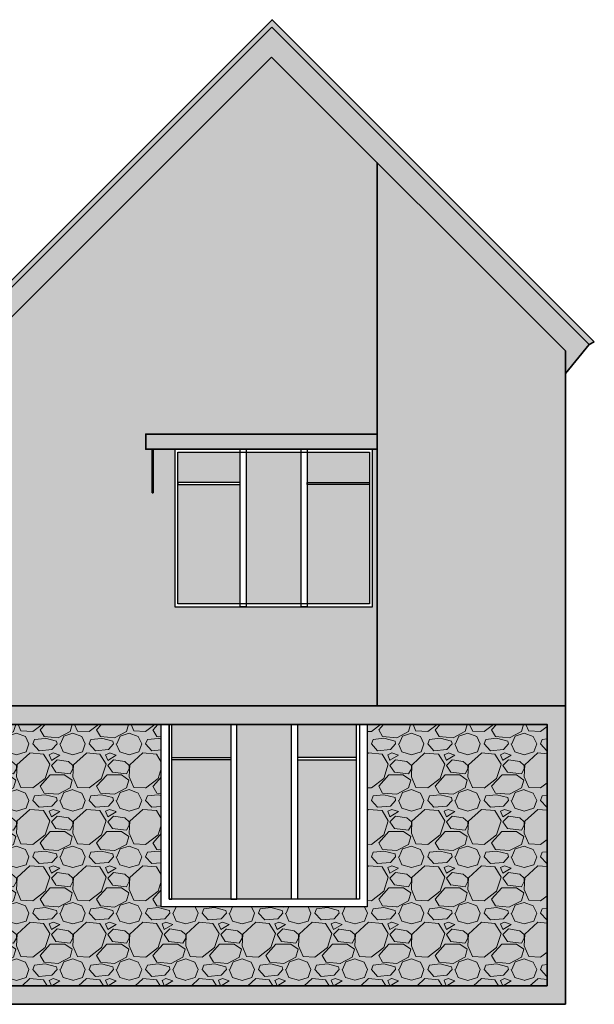
# Model space of a CAD drawing. Units: feet. Extents: x 2613 to 3913, y 950 to 1393.
# Tile 5 of 6: x 2948 to 3207, y 950 to 1393. Entities that reach past the tile are written whole.
import ezdxf

# ---------------------------------------------------------------- set-up
doc = ezdxf.new("R2010")
doc.units = ezdxf.units.FT
for name, color, linetype, lineweight in [('A-ELEV', 7, 'Continuous', 35), ('A-ELEV-PATT', 9, 'Continuous', 13), ('A-FLOR-STRS', 7, 'Continuous', 25), ('A-GLAZ', 4, 'Continuous', 25), ('A-ROOF', 1, 'Continuous', 35)]:
    doc.layers.add(name, color=color, linetype=linetype, lineweight=lineweight)

msp = doc.modelspace()

# ---------------------------------------------------------------- hatches: boundary and pattern name
at = {"layer": 'A-ELEV-PATT'}
h = msp.add_hatch(color=256, dxfattribs=at)
h.dxf.hatch_style = 1
h.paths.add_polyline_path([(3108.91, 1328.81), (3061.44, 1376.28), (2929.45, 1244.29), (2929.45, 1223.38), (2942.09, 1223.38), (2942.09, 1215.5), (2929.45, 1215.5), (2929.45, 1084.12), (3108.91, 1084.12), (3108.91, 1199.69), (3106.87, 1199.69), (3106.87, 1128.72), (3017.91, 1128.72), (3017.91, 1199.69), (3008.08, 1199.69), (3008.08, 1180.01), (3007.65, 1180.01), (3007.65, 1199.69), (3004.75, 1199.69), (3004.75, 1206.47), (3108.91, 1206.47)])
h.paths.add_polyline_path([(3061.44, 1376.28), (3193.8, 1243.92), (3193.8, 1233.84), (3204.34, 1246.9), (3061.54, 1389.71), (2918.82, 1247), (2929.45, 1233.69), (2929.45, 1244.29)])
h.paths.add_polyline_path([(3061.54, 1389.71), (3204.34, 1246.9), (3206.69, 1248.02), (3061.63, 1393.09), (2916.59, 1248.06), (2918.82, 1247)])
h.paths.add_polyline_path([(2925.65, 1257.12), (2667.59, 1257.12), (2651.33, 1257.12), (2651.33, 1252.28), (2920.82, 1252.28)])
h.paths.add_polyline_path([(2920.82, 1252.28), (2651.33, 1252.28, -0.144454), (2652.15, 1251.12), (2667.59, 1251.12), (2919.65, 1251.12)])
h.paths.add_polyline_path([(2918.82, 1247), (2916.59, 1248.06), (2919.65, 1251.12), (2667.59, 1251.12), (2652.15, 1251.12), (2667.59, 1229.14), (2667.59, 1233.69), (2929.45, 1233.69)])
h.paths.add_polyline_path([(2710.6, 1223.38), (2929.45, 1223.38), (2929.45, 1233.69), (2667.59, 1233.69), (2667.59, 1229.14), (2667.59, 1201.16), (2720.67, 1201.16), (2710.6, 1215.5)])
h.paths.add_polyline_path([(2942.09, 1223.38), (2710.6, 1223.38), (2710.6, 1215.5), (2921.48, 1215.5), (2942.09, 1215.5)])
h.paths.add_polyline_path([(2929.45, 1215.5), (2921.48, 1215.5), (2710.6, 1215.5), (2733.47, 1182.94), (2733.47, 1195.74), (2741.22, 1195.74), (2929.45, 1195.74)])
h.paths.add_polyline_path([(2721, 1200.68), (2661.89, 1200.68), (2661.89, 1195.74), (2724.47, 1195.74)])
h.paths.add_polyline_path([(2733.47, 1182.94), (2727.27, 1191.76), (2727.27, 1133.88), (2731.7, 1133.88), (2731.7, 1169.74), (2731.61, 1169.74), (2731.61, 1170.13), (2733.47, 1170.13)])
h.paths.add_polyline_path([(2929.45, 1183.04), (2741.22, 1183.04), (2741.22, 1170.13), (2743.07, 1170.13), (2743.07, 1169.74), (2743.07, 1112.32), (2759.57, 1112.32), (2759.57, 1167.82), (2763.7, 1167.82), (2763.7, 1112.32), (2781.75, 1112.32), (2781.75, 1167.82), (2785.87, 1167.82), (2785.87, 1112.32), (2803.92, 1112.32), (2803.92, 1167.82), (2808.05, 1167.82), (2808.05, 1112.32), (2826.09, 1112.32), (2826.09, 1167.82), (2830.22, 1167.82), (2830.22, 1112.32), (2875.17, 1112.32), (2875.17, 1171.49), (2929.45, 1171.49)])
h.paths.add_polyline_path([(2731.7, 1133.88), (2661.89, 1133.88), (2661.89, 1084.12), (2730.99, 1084.12), (2730.99, 1112.32), (2731.7, 1112.32)])
h.paths.add_polyline_path([(2929.45, 1112.32), (2730.99, 1112.32), (2730.99, 1084.12), (2929.45, 1084.12)])
h.paths.add_polyline_path([(2929.45, 1084.12), (2730.99, 1084.12), (2661.89, 1084.12), (2612.72, 1084.12), (2612.72, 1082.68), (2929.45, 1082.68)])
h.paths.add_polyline_path([(2929.45, 1082.68), (2612.72, 1082.68), (2639.32, 1062.44), (2733.47, 1062.44), (2733.47, 1063.35), (2639.62, 1063.35), (2615.43, 1081.77), (2723.91, 1081.77), (2739.71, 1069.74), (2741.22, 1069.74), (2725.42, 1081.77), (2929.45, 1081.77)])
h.paths.add_polyline_path([(2671.42, 1081.77), (2668.07, 1081.77), (2692.27, 1063.35), (2695.62, 1063.35)], flags=17)
h.paths.add_polyline_path([(2741.22, 1069.74), (2741.22, 1068.59), (2748.11, 1063.35), (2741.22, 1063.35), (2741.22, 1062.44), (2750.82, 1062.44)], flags=17)
h.paths.add_polyline_path([(2929.45, 1081.77), (2725.42, 1081.77), (2750.82, 1062.44), (2741.22, 1062.44), (2741.22, 1047.95), (2743.07, 1047.95), (2743.07, 1047.56), (2743.07, 967.97), (2875.17, 967.97), (2875.17, 1066.37), (2929.45, 1066.37)])
h.paths.add_polyline_path([(2778.55, 1066.37), (2806.94, 1066.37), (2806.94, 982.04), (2778.55, 982.04)], flags=16)
h.paths.add_polyline_path([(2778.55, 1064.05), (2806.94, 1064.05), (2806.94, 1063.39), (2778.55, 1063.39)], flags=16)
h.paths.add_polyline_path([(2778.55, 1061.07), (2806.94, 1061.07), (2806.94, 1060.41), (2778.55, 1060.41)], flags=0)
h.paths.add_polyline_path([(2778.55, 1058.09), (2806.94, 1058.09), (2806.94, 1057.43), (2778.55, 1057.43)], flags=0)
h.paths.add_polyline_path([(2778.55, 1055.11), (2806.94, 1055.11), (2806.94, 1054.45), (2778.55, 1054.45)], flags=0)
h.paths.add_polyline_path([(2778.55, 1052.13), (2806.94, 1052.13), (2806.94, 1051.47), (2778.55, 1051.47)], flags=0)
h.paths.add_polyline_path([(2778.55, 1049.15), (2806.94, 1049.15), (2806.94, 1048.49), (2778.55, 1048.49)], flags=0)
h.paths.add_polyline_path([(2778.55, 1046.18), (2806.94, 1046.18), (2806.94, 1045.51), (2778.55, 1045.51)], flags=0)
h.paths.add_polyline_path([(2778.55, 1043.2), (2806.94, 1043.2), (2806.94, 1042.53), (2778.55, 1042.53)], flags=0)
h.paths.add_polyline_path([(2778.55, 1040.22), (2806.94, 1040.22), (2806.94, 1039.56), (2778.55, 1039.56)], flags=0)
h.paths.add_polyline_path([(2778.55, 1037.24), (2806.94, 1037.24), (2806.94, 1036.58), (2778.55, 1036.58)], flags=0)
h.paths.add_polyline_path([(2778.55, 1034.26), (2806.94, 1034.26), (2806.94, 1033.6), (2778.55, 1033.6)], flags=0)
h.paths.add_polyline_path([(2778.55, 1031.28), (2806.94, 1031.28), (2806.94, 1030.62), (2778.55, 1030.62)], flags=0)
h.paths.add_polyline_path([(2778.55, 1028.3), (2806.94, 1028.3), (2806.94, 1027.64), (2778.55, 1027.64)], flags=0)
h.paths.add_polyline_path([(2778.55, 1025.32), (2806.94, 1025.32), (2806.94, 1024.66), (2778.55, 1024.66)], flags=0)
h.paths.add_polyline_path([(2778.55, 1022.34), (2806.94, 1022.34), (2806.94, 1021.68), (2778.55, 1021.68)], flags=0)
h.paths.add_polyline_path([(2778.55, 1019.36), (2806.94, 1019.36), (2806.94, 1018.7), (2778.55, 1018.7)], flags=0)
h.paths.add_polyline_path([(2778.55, 1016.71), (2806.94, 1016.71), (2806.94, 1016.05), (2778.55, 1016.05)], flags=0)
h.paths.add_polyline_path([(2824.02, 1066.37), (2852.41, 1066.37), (2852.41, 982.04), (2824.02, 982.04)], flags=16)
h.paths.add_polyline_path([(2778.55, 1014.07), (2806.94, 1014.07), (2806.94, 1013.4), (2778.55, 1013.4)], flags=0)
h.paths.add_polyline_path([(2824.02, 1064.05), (2852.41, 1064.05), (2852.41, 1063.39), (2824.02, 1063.39)], flags=16)
h.paths.add_polyline_path([(2824.02, 1061.07), (2852.41, 1061.07), (2852.41, 1060.41), (2824.02, 1060.41)], flags=0)
h.paths.add_polyline_path([(2824.02, 1058.09), (2852.41, 1058.09), (2852.41, 1057.43), (2824.02, 1057.43)], flags=0)
h.paths.add_polyline_path([(2824.02, 1055.11), (2852.41, 1055.11), (2852.41, 1054.45), (2824.02, 1054.45)], flags=16)
h.paths.add_polyline_path([(2824.02, 1052.13), (2852.41, 1052.13), (2852.41, 1051.47), (2824.02, 1051.47)], flags=0)
h.paths.add_polyline_path([(2778.55, 1011.09), (2806.94, 1011.09), (2806.94, 1010.43), (2778.55, 1010.43)], flags=0)
h.paths.add_polyline_path([(2824.02, 1049.15), (2852.41, 1049.15), (2852.41, 1048.49), (2824.02, 1048.49)], flags=0)
h.paths.add_polyline_path([(2824.02, 1046.18), (2852.41, 1046.18), (2852.41, 1045.51), (2824.02, 1045.51)], flags=0)
h.paths.add_polyline_path([(2824.02, 1043.2), (2852.41, 1043.2), (2852.41, 1042.53), (2824.02, 1042.53)], flags=0)
h.paths.add_polyline_path([(2778.55, 1008.11), (2806.94, 1008.11), (2806.94, 1007.45), (2778.55, 1007.45)], flags=0)
h.paths.add_polyline_path([(2824.02, 1040.22), (2852.41, 1040.22), (2852.41, 1039.56), (2824.02, 1039.56)], flags=0)
h.paths.add_polyline_path([(2824.02, 1037.24), (2852.41, 1037.24), (2852.41, 1036.58), (2824.02, 1036.58)], flags=0)
h.paths.add_polyline_path([(2778.55, 1005.13), (2806.94, 1005.13), (2806.94, 1004.47), (2778.55, 1004.47)], flags=0)
h.paths.add_polyline_path([(2824.02, 1034.26), (2852.41, 1034.26), (2852.41, 1033.6), (2824.02, 1033.6)], flags=0)
h.paths.add_polyline_path([(2824.02, 1031.28), (2852.41, 1031.28), (2852.41, 1030.62), (2824.02, 1030.62)], flags=0)
h.paths.add_polyline_path([(2778.55, 1002.15), (2806.94, 1002.15), (2806.94, 1001.49), (2778.55, 1001.49)], flags=0)
h.paths.add_polyline_path([(2824.02, 1028.3), (2852.41, 1028.3), (2852.41, 1027.64), (2824.02, 1027.64)], flags=0)
h.paths.add_polyline_path([(2778.55, 999.17), (2806.94, 999.17), (2806.94, 998.51), (2778.55, 998.51)], flags=0)
h.paths.add_polyline_path([(2824.02, 1025.32), (2852.41, 1025.32), (2852.41, 1024.66), (2824.02, 1024.66)], flags=0)
h.paths.add_polyline_path([(2824.02, 1022.34), (2852.41, 1022.34), (2852.41, 1021.68), (2824.02, 1021.68)], flags=0)
h.paths.add_polyline_path([(2778.55, 996.19), (2806.94, 996.19), (2806.94, 995.53), (2778.55, 995.53)], flags=0)
h.paths.add_polyline_path([(2824.02, 1019.36), (2852.41, 1019.36), (2852.41, 1018.7), (2824.02, 1018.7)], flags=0)
h.paths.add_polyline_path([(2778.55, 993.21), (2806.94, 993.21), (2806.94, 992.55), (2778.55, 992.55)], flags=0)
h.paths.add_polyline_path([(2824.02, 1016.38), (2852.41, 1016.38), (2852.41, 1015.72), (2824.02, 1015.72)], flags=0)
h.paths.add_polyline_path([(2824.02, 1013.4), (2852.41, 1013.4), (2852.41, 1012.74), (2824.02, 1012.74)], flags=0)
h.paths.add_polyline_path([(2778.55, 990.23), (2806.94, 990.23), (2806.94, 989.57), (2778.55, 989.57)], flags=0)
h.paths.add_polyline_path([(2824.02, 1010.43), (2852.41, 1010.43), (2852.41, 1009.76), (2824.02, 1009.76)], flags=0)
h.paths.add_polyline_path([(2778.55, 987.25), (2806.94, 987.25), (2806.94, 986.59), (2778.55, 986.59)], flags=0)
h.paths.add_polyline_path([(2824.02, 1007.45), (2852.41, 1007.45), (2852.41, 1006.78), (2824.02, 1006.78)], flags=0)
h.paths.add_polyline_path([(2778.55, 984.27), (2806.94, 984.27), (2806.94, 983.61), (2778.55, 983.61)], flags=0)
h.paths.add_polyline_path([(2824.02, 1004.47), (2852.41, 1004.47), (2852.41, 1003.81), (2824.02, 1003.81)], flags=0)
h.paths.add_polyline_path([(2824.02, 1001.49), (2852.41, 1001.49), (2852.41, 1000.83), (2824.02, 1000.83)], flags=0)
h.paths.add_polyline_path([(2824.02, 998.51), (2852.41, 998.51), (2852.41, 997.85), (2824.02, 997.85)], flags=0)
h.paths.add_polyline_path([(2824.02, 995.53), (2852.41, 995.53), (2852.41, 994.87), (2824.02, 994.87)], flags=0)
h.paths.add_polyline_path([(2824.02, 992.55), (2852.41, 992.55), (2852.41, 991.89), (2824.02, 991.89)], flags=0)
h.paths.add_polyline_path([(2824.02, 989.57), (2852.41, 989.57), (2852.41, 988.91), (2824.02, 988.91)], flags=0)
h.paths.add_polyline_path([(2824.02, 986.59), (2852.41, 986.59), (2852.41, 985.93), (2824.02, 985.93)], flags=0)
h.paths.add_polyline_path([(2824.02, 983.61), (2852.41, 983.61), (2852.41, 982.95), (2824.02, 982.95)], flags=0)
h.paths.add_polyline_path([(2731.7, 1047.56), (2731.61, 1047.56), (2731.61, 1047.95), (2733.47, 1047.95), (2733.47, 1062.44), (2727.27, 1062.44), (2727.27, 1000.58), (2667.59, 1000.58), (2667.59, 1062.44), (2664.87, 1062.44), (2664.87, 965.01), (2730.76, 964.93), (2730.76, 967.97), (2731.7, 967.97)])
h.paths.add_polyline_path([(2728.06, 961.9), (2730.76, 961.9), (2730.76, 964.93), (2663.94, 964.93), (2663.94, 949.74), (2725.36, 949.74), (2725.36, 955.82), (2728.06, 955.82)])
h.paths.add_polyline_path([(2929.45, 967.97), (2730.76, 967.97), (2730.76, 961.9), (2929.45, 961.9)])
h.paths.add_polyline_path([(2929.45, 961.9), (2730.76, 961.9), (2728.06, 961.9), (2728.06, 955.82), (2929.45, 955.82)])
h.paths.add_polyline_path([(2929.45, 955.82), (2728.06, 955.82), (2725.36, 955.82), (2725.36, 949.74), (2929.45, 949.74)])
h.paths.add_polyline_path([(2741.22, 1069.74), (2733.47, 1069.74), (2733.47, 1047.95), (2741.22, 1047.95)], flags=17)
h.paths.add_polyline_path([(2741.22, 1195.74), (2733.47, 1195.74), (2733.47, 1182.94), (2733.47, 1170.13), (2741.22, 1170.13), (2741.22, 1183.04)])
h.paths.add_polyline_path([(3193.8, 1084.12), (2929.45, 1084.12), (2929.45, 1082.68), (2929.45, 1081.77), (2929.45, 1066.37), (2929.45, 949.74), (3193.8, 949.74)])
h.paths.add_polyline_path([(2937.79, 1075.78), (3185.46, 1075.78), (3185.46, 958.09), (2937.79, 958.09)], flags=16)
h.paths.add_polyline_path([(3011.76, 1075.78), (3104.46, 1075.78), (3104.46, 993.6), (3011.76, 993.6)], flags=0)
h.paths.add_polyline_path([(3015.24, 1075.78), (3016.57, 1075.78), (3016.57, 1060.85), (3043.1, 1060.85), (3043.1, 1075.78), (3045.77, 1075.78), (3045.77, 997.08), (3070.45, 997.08), (3070.45, 1075.78), (3073.12, 1075.78), (3073.12, 1060.85), (3099.64, 1060.85), (3099.64, 1075.78), (3100.98, 1075.78), (3100.98, 997.08), (3099.64, 997.08), (3015.24, 997.08)], flags=0)
h = msp.add_hatch(color=256, dxfattribs=at)
h.dxf.hatch_style = 1
h.paths.add_polyline_path([(3108.91, 1328.81), (3108.91, 1084.12), (3193.8, 1084.12), (3193.8, 1243.92)])
h = msp.add_hatch(color=256, dxfattribs=at)
h.dxf.hatch_style = 1
h.paths.add_polyline_path([(3108.91, 1206.47), (3004.75, 1206.47), (3004.75, 1199.69), (3108.91, 1199.69)])
h = msp.add_hatch(color=256, dxfattribs=at)
h.dxf.hatch_style = 1
h.paths.add_polyline_path([(2768.1, 1195.09), (2741.95, 1195.09), (2741.95, 1183.7), (2768.1, 1183.7)])
h.paths.add_polyline_path([(2794.91, 1195.09), (2768.76, 1195.09), (2768.76, 1183.7), (2794.91, 1183.7)])
h.paths.add_polyline_path([(2821.72, 1195.09), (2795.57, 1195.09), (2795.57, 1183.7), (2821.72, 1183.7)])
h.paths.add_polyline_path([(2848.53, 1195.09), (2822.38, 1195.09), (2822.38, 1183.7), (2848.53, 1183.7)])
h.paths.add_polyline_path([(2875.34, 1195.09), (2849.19, 1195.09), (2849.19, 1183.7), (2875.34, 1183.7)])
h.paths.add_polyline_path([(2683.29, 1193.04), (2670.29, 1193.04), (2670.29, 1190.17), (2683.29, 1190.17)])
h.paths.add_polyline_path([(2696.31, 1193.04), (2683.32, 1193.04), (2683.32, 1190.17), (2696.31, 1190.17)])
h.paths.add_polyline_path([(2696.31, 1190.14), (2683.32, 1190.14), (2683.32, 1187.27), (2696.31, 1187.27)])
h.paths.add_polyline_path([(2683.29, 1190.14), (2670.29, 1190.14), (2670.29, 1187.27), (2683.29, 1187.27)])
h.paths.add_polyline_path([(2683.29, 1187.24), (2670.29, 1187.24), (2670.29, 1184.37), (2683.29, 1184.37)])
h.paths.add_polyline_path([(2696.31, 1187.24), (2683.32, 1187.24), (2683.32, 1184.37), (2696.31, 1184.37)])
h.paths.add_polyline_path([(2683.29, 1184.34), (2670.29, 1184.34), (2670.29, 1181.47), (2683.29, 1181.47)])
h.paths.add_polyline_path([(2696.31, 1184.34), (2683.32, 1184.34), (2683.32, 1181.47), (2696.31, 1181.47)])
h.paths.add_polyline_path([(2683.29, 1181.44), (2670.29, 1181.44), (2670.29, 1178.57), (2683.29, 1178.57)])
h.paths.add_polyline_path([(2696.31, 1181.44), (2683.32, 1181.44), (2683.32, 1178.57), (2696.31, 1178.57)])
h.paths.add_polyline_path([(2696.31, 1178.53), (2683.32, 1178.53), (2683.32, 1175.67), (2696.31, 1175.67)])
h.paths.add_polyline_path([(2683.29, 1178.53), (2670.29, 1178.53), (2670.29, 1175.67), (2683.29, 1175.67)])
h.paths.add_polyline_path([(2683.29, 1175.63), (2670.29, 1175.63), (2670.29, 1172.76), (2683.29, 1172.76)])
h.paths.add_polyline_path([(2696.31, 1175.63), (2683.32, 1175.63), (2683.32, 1172.76), (2696.31, 1172.76)])
h.paths.add_polyline_path([(2683.29, 1172.73), (2670.29, 1172.73), (2670.29, 1169.86), (2683.29, 1169.86)])
h.paths.add_polyline_path([(2696.31, 1172.73), (2683.32, 1172.73), (2683.32, 1169.86), (2696.31, 1169.86)])
h.paths.add_polyline_path([(2696.31, 1169.83), (2683.32, 1169.83), (2683.32, 1166.96), (2696.31, 1166.96)])
h.paths.add_polyline_path([(2683.29, 1169.83), (2670.29, 1169.83), (2670.29, 1166.96), (2683.29, 1166.96)])
h.paths.add_polyline_path([(2696.31, 1166.93), (2683.32, 1166.93), (2683.32, 1164.06), (2696.31, 1164.06)])
h.paths.add_polyline_path([(2683.29, 1166.93), (2670.29, 1166.93), (2670.29, 1164.06), (2683.29, 1164.06)])
h.paths.add_polyline_path([(2683.29, 1164.03), (2670.29, 1164.03), (2670.29, 1161.16), (2683.29, 1161.16)])
h.paths.add_polyline_path([(2696.31, 1164.03), (2683.32, 1164.03), (2683.32, 1161.16), (2696.31, 1161.16)])
h.paths.add_polyline_path([(2696.31, 1161.12), (2683.32, 1161.12), (2683.32, 1158.25), (2696.31, 1158.25)])
h.paths.add_polyline_path([(2683.29, 1161.12), (2670.29, 1161.12), (2670.29, 1158.25), (2683.29, 1158.25)])
h.paths.add_polyline_path([(2683.29, 1158.22), (2670.29, 1158.22), (2670.29, 1155.35), (2683.29, 1155.35)])
h.paths.add_polyline_path([(2696.31, 1158.22), (2683.32, 1158.22), (2683.32, 1155.35), (2696.31, 1155.35)])
h.paths.add_polyline_path([(2696.31, 1155.32), (2683.32, 1155.32), (2683.32, 1152.45), (2696.31, 1152.45)])
h.paths.add_polyline_path([(2683.29, 1155.32), (2670.29, 1155.32), (2670.29, 1152.45), (2683.29, 1152.45)])
h.paths.add_polyline_path([(2683.29, 1152.42), (2670.29, 1152.42), (2670.29, 1149.55), (2683.29, 1149.55)])
h.paths.add_polyline_path([(2696.31, 1152.42), (2683.32, 1152.42), (2683.32, 1149.55), (2696.31, 1149.55)])
h.paths.add_polyline_path([(2683.29, 1149.52), (2670.29, 1149.52), (2670.29, 1146.65), (2683.29, 1146.65)])
h.paths.add_polyline_path([(2696.31, 1149.52), (2683.32, 1149.52), (2683.32, 1146.65), (2696.31, 1146.65)])
h.paths.add_polyline_path([(2696.31, 1146.61), (2683.32, 1146.61), (2683.32, 1143.75), (2696.31, 1143.75)])
h.paths.add_polyline_path([(2683.29, 1146.61), (2670.29, 1146.61), (2670.29, 1143.75), (2683.29, 1143.75)])
h.paths.add_polyline_path([(2683.29, 1143.71), (2670.29, 1143.71), (2670.29, 1140.84), (2683.29, 1140.84)])
h.paths.add_polyline_path([(2696.31, 1143.71), (2683.32, 1143.71), (2683.32, 1140.84), (2696.31, 1140.84)])
h.paths.add_polyline_path([(2683.29, 1140.81), (2670.29, 1140.81), (2670.29, 1137.94), (2683.29, 1137.94)])
h.paths.add_polyline_path([(2696.31, 1140.81), (2683.32, 1140.81), (2683.32, 1137.94), (2696.31, 1137.94)])
h.paths.add_polyline_path([(2683.29, 1137.91), (2670.29, 1137.91), (2670.29, 1136.58), (2683.29, 1136.58)])
h.paths.add_polyline_path([(2696.31, 1137.91), (2683.32, 1137.91), (2683.32, 1136.58), (2696.31, 1136.58)])
h.paths.add_polyline_path([(3074.7, 1198.4), (3050.02, 1198.4), (3050.02, 1130.01), (3074.7, 1130.01)])
h.paths.add_polyline_path([(3047.34, 1198.4), (3019.29, 1198.4), (3019.29, 1184.76), (3047.34, 1184.76)])
h.paths.add_polyline_path([(3047.34, 1183.78), (3019.29, 1183.78), (3019.29, 1130.01), (3047.34, 1130.01)])
h.paths.add_polyline_path([(3105.48, 1198.4), (3077.37, 1198.4), (3077.37, 1184.76), (3105.48, 1184.76)])
h.paths.add_polyline_path([(3105.48, 1183.78), (3077.37, 1183.78), (3077.37, 1130.01), (3105.48, 1130.01)])
h.paths.add_polyline_path([(3070.45, 1075.78), (3045.77, 1075.78), (3045.77, 997.08), (3070.45, 997.08)])
h.paths.add_polyline_path([(3099.64, 1075.78), (3073.12, 1075.78), (3073.12, 1060.85), (3099.64, 1060.85)])
h.paths.add_polyline_path([(3099.64, 1059.87), (3073.12, 1059.87), (3073.12, 997.08), (3099.64, 997.08)])
h.paths.add_polyline_path([(3043.1, 1075.78), (3016.57, 1075.78), (3016.57, 1060.85), (3043.1, 1060.85)])
h.paths.add_polyline_path([(3043.1, 1059.87), (3016.57, 1059.87), (3016.57, 997.08), (3043.1, 997.08)])
h.paths.add_polyline_path([(2683.29, 1059.73), (2670.29, 1059.73), (2670.29, 1056.87), (2683.29, 1056.87)])
h.paths.add_polyline_path([(2696.31, 1059.73), (2683.32, 1059.73), (2683.32, 1056.87), (2696.31, 1056.87)])
h.paths.add_polyline_path([(2696.31, 1056.83), (2683.32, 1056.83), (2683.32, 1053.96), (2696.31, 1053.96)])
h.paths.add_polyline_path([(2683.29, 1056.83), (2670.29, 1056.83), (2670.29, 1053.96), (2683.29, 1053.96)])
h.paths.add_polyline_path([(2683.29, 1053.93), (2670.29, 1053.93), (2670.29, 1051.06), (2683.29, 1051.06)])
h.paths.add_polyline_path([(2696.31, 1053.93), (2683.32, 1053.93), (2683.32, 1051.06), (2696.31, 1051.06)])
h.paths.add_polyline_path([(2683.29, 1051.03), (2670.29, 1051.03), (2670.29, 1048.16), (2683.29, 1048.16)])
h.paths.add_polyline_path([(2696.31, 1051.03), (2683.32, 1051.03), (2683.32, 1048.16), (2696.31, 1048.16)])
h.paths.add_polyline_path([(2683.29, 1048.13), (2670.29, 1048.13), (2670.29, 1045.26), (2683.29, 1045.26)])
h.paths.add_polyline_path([(2696.31, 1048.13), (2683.32, 1048.13), (2683.32, 1045.26), (2696.31, 1045.26)])
h.paths.add_polyline_path([(2696.31, 1045.23), (2683.32, 1045.23), (2683.32, 1042.36), (2696.31, 1042.36)])
h.paths.add_polyline_path([(2683.29, 1045.23), (2670.29, 1045.23), (2670.29, 1042.36), (2683.29, 1042.36)])
h.paths.add_polyline_path([(2683.29, 1042.32), (2670.29, 1042.32), (2670.29, 1039.46), (2683.29, 1039.46)])
h.paths.add_polyline_path([(2696.31, 1042.32), (2683.32, 1042.32), (2683.32, 1039.46), (2696.31, 1039.46)])
h.paths.add_polyline_path([(2696.31, 1039.42), (2683.32, 1039.42), (2683.32, 1036.55), (2696.31, 1036.55)])
h.paths.add_polyline_path([(2683.29, 1039.42), (2670.29, 1039.42), (2670.29, 1036.55), (2683.29, 1036.55)])
h.paths.add_polyline_path([(2683.29, 1036.52), (2670.29, 1036.52), (2670.29, 1033.65), (2683.29, 1033.65)])
h.paths.add_polyline_path([(2696.31, 1036.52), (2683.32, 1036.52), (2683.32, 1033.65), (2696.31, 1033.65)])
h.paths.add_polyline_path([(2696.31, 1033.62), (2683.32, 1033.62), (2683.32, 1030.75), (2696.31, 1030.75)])
h.paths.add_polyline_path([(2683.29, 1033.62), (2670.29, 1033.62), (2670.29, 1030.75), (2683.29, 1030.75)])
h.paths.add_polyline_path([(2696.31, 1030.72), (2683.32, 1030.72), (2683.32, 1027.85), (2696.31, 1027.85)])
h.paths.add_polyline_path([(2683.29, 1030.72), (2670.29, 1030.72), (2670.29, 1027.85), (2683.29, 1027.85)])
h.paths.add_polyline_path([(2683.29, 1027.82), (2670.29, 1027.82), (2670.29, 1024.95), (2683.29, 1024.95)])
h.paths.add_polyline_path([(2696.31, 1027.82), (2683.32, 1027.82), (2683.32, 1024.95), (2696.31, 1024.95)])
h.paths.add_polyline_path([(2696.31, 1024.91), (2683.32, 1024.91), (2683.32, 1022.05), (2696.31, 1022.05)])
h.paths.add_polyline_path([(2683.29, 1024.91), (2670.29, 1024.91), (2670.29, 1022.05), (2683.29, 1022.05)])
h.paths.add_polyline_path([(2683.29, 1022.01), (2670.29, 1022.01), (2670.29, 1019.14), (2683.29, 1019.14)])
h.paths.add_polyline_path([(2696.31, 1022.01), (2683.32, 1022.01), (2683.32, 1019.14), (2696.31, 1019.14)])
h.paths.add_polyline_path([(2696.31, 1019.11), (2683.32, 1019.11), (2683.32, 1016.24), (2696.31, 1016.24)])
h.paths.add_polyline_path([(2683.29, 1019.11), (2670.29, 1019.11), (2670.29, 1016.24), (2683.29, 1016.24)])
h.paths.add_polyline_path([(2683.29, 1016.21), (2670.29, 1016.21), (2670.29, 1013.34), (2683.29, 1013.34)])
h.paths.add_polyline_path([(2696.31, 1016.21), (2683.32, 1016.21), (2683.32, 1013.34), (2696.31, 1013.34)])
h.paths.add_polyline_path([(2696.31, 1013.31), (2683.32, 1013.31), (2683.32, 1010.44), (2696.31, 1010.44)])
h.paths.add_polyline_path([(2683.29, 1013.31), (2670.29, 1013.31), (2670.29, 1010.44), (2683.29, 1010.44)])
h.paths.add_polyline_path([(2683.29, 1010.41), (2670.29, 1010.41), (2670.29, 1007.54), (2683.29, 1007.54)])
h.paths.add_polyline_path([(2696.31, 1010.41), (2683.32, 1010.41), (2683.32, 1007.54), (2696.31, 1007.54)])
h.paths.add_polyline_path([(2696.31, 1007.5), (2683.32, 1007.5), (2683.32, 1004.64), (2696.31, 1004.64)])
h.paths.add_polyline_path([(2683.29, 1007.5), (2670.29, 1007.5), (2670.29, 1004.64), (2683.29, 1004.64)])
h.paths.add_polyline_path([(2683.29, 1004.6), (2670.29, 1004.6), (2670.29, 1003.28), (2683.29, 1003.28)])
h.paths.add_polyline_path([(2696.31, 1004.6), (2683.32, 1004.6), (2683.32, 1003.28), (2696.31, 1003.28)])
h.paths.add_polyline_path([(2806.94, 1066.37), (2778.55, 1066.37), (2778.55, 1064.05), (2806.94, 1064.05)])
h.paths.add_polyline_path([(2806.94, 1063.39), (2778.55, 1063.39), (2778.55, 1061.07), (2806.94, 1061.07)])
h.paths.add_polyline_path([(2806.94, 1060.41), (2778.55, 1060.41), (2778.55, 1058.09), (2806.94, 1058.09)])
h.paths.add_polyline_path([(2806.94, 1057.43), (2778.55, 1057.43), (2778.55, 1055.11), (2806.94, 1055.11)])
h.paths.add_polyline_path([(2806.94, 1054.45), (2778.55, 1054.45), (2778.55, 1052.13), (2806.94, 1052.13)])
h.paths.add_polyline_path([(2806.94, 1051.47), (2778.55, 1051.47), (2778.55, 1049.15), (2806.94, 1049.15)])
h.paths.add_polyline_path([(2806.94, 1048.49), (2778.55, 1048.49), (2778.55, 1046.18), (2806.94, 1046.18)])
h.paths.add_polyline_path([(2806.94, 1045.51), (2778.55, 1045.51), (2778.55, 1043.2), (2806.94, 1043.2)])
h.paths.add_polyline_path([(2806.94, 1042.53), (2778.55, 1042.53), (2778.55, 1040.22), (2806.94, 1040.22)])
h.paths.add_polyline_path([(2806.94, 1039.56), (2778.55, 1039.56), (2778.55, 1037.24), (2806.94, 1037.24)])
h.paths.add_polyline_path([(2806.94, 1036.58), (2778.55, 1036.58), (2778.55, 1034.26), (2806.94, 1034.26)])
h.paths.add_polyline_path([(2806.94, 1033.6), (2778.55, 1033.6), (2778.55, 1031.28), (2806.94, 1031.28)])
h.paths.add_polyline_path([(2806.94, 1030.62), (2778.55, 1030.62), (2778.55, 1028.3), (2806.94, 1028.3)])
h.paths.add_polyline_path([(2806.94, 1027.64), (2778.55, 1027.64), (2778.55, 1025.32), (2806.94, 1025.32)])
h.paths.add_polyline_path([(2806.94, 1024.66), (2778.55, 1024.66), (2778.55, 1022.34), (2806.94, 1022.34)])
h.paths.add_polyline_path([(2806.94, 1021.68), (2778.55, 1021.68), (2778.55, 1019.36), (2806.94, 1019.36)])
h.paths.add_polyline_path([(2806.94, 1018.7), (2778.55, 1018.7), (2778.55, 1016.71), (2806.94, 1016.71)])
h.paths.add_polyline_path([(2806.94, 1016.05), (2778.55, 1016.05), (2778.55, 1014.07), (2806.94, 1014.07)])
h.paths.add_polyline_path([(2806.94, 1013.4), (2778.55, 1013.4), (2778.55, 1011.09), (2806.94, 1011.09)])
h.paths.add_polyline_path([(2806.94, 1010.43), (2778.55, 1010.43), (2778.55, 1008.11), (2806.94, 1008.11)])
h.paths.add_polyline_path([(2806.94, 1007.45), (2778.55, 1007.45), (2778.55, 1005.13), (2806.94, 1005.13)])
h.paths.add_polyline_path([(2806.94, 1004.47), (2778.55, 1004.47), (2778.55, 1002.15), (2806.94, 1002.15)])
h.paths.add_polyline_path([(2806.94, 1001.49), (2778.55, 1001.49), (2778.55, 999.17), (2806.94, 999.17)])
h.paths.add_polyline_path([(2806.94, 998.51), (2778.55, 998.51), (2778.55, 996.19), (2806.94, 996.19)])
h.paths.add_polyline_path([(2806.94, 983.61), (2778.55, 983.61), (2778.55, 982.04), (2806.94, 982.04)])
h.paths.add_polyline_path([(2806.94, 986.59), (2778.55, 986.59), (2778.55, 984.27), (2806.94, 984.27)])
h.paths.add_polyline_path([(2806.94, 989.57), (2778.55, 989.57), (2778.55, 987.25), (2806.94, 987.25)])
h.paths.add_polyline_path([(2806.94, 992.55), (2778.55, 992.55), (2778.55, 990.23), (2806.94, 990.23)])
h.paths.add_polyline_path([(2806.94, 995.53), (2778.55, 995.53), (2778.55, 993.21), (2806.94, 993.21)])
h.paths.add_polyline_path([(2852.41, 985.93), (2824.02, 985.93), (2824.02, 983.61), (2852.41, 983.61)])
h.paths.add_polyline_path([(2852.41, 982.95), (2824.02, 982.95), (2824.02, 982.04), (2852.41, 982.04)])
h.paths.add_polyline_path([(2852.41, 988.91), (2824.02, 988.91), (2824.02, 986.59), (2852.41, 986.59)])
h.paths.add_polyline_path([(2852.41, 991.89), (2824.02, 991.89), (2824.02, 989.57), (2852.41, 989.57)])
h.paths.add_polyline_path([(2852.41, 994.87), (2824.02, 994.87), (2824.02, 992.55), (2852.41, 992.55)])
h.paths.add_polyline_path([(2852.41, 997.85), (2824.02, 997.85), (2824.02, 995.53), (2852.41, 995.53)])
h.paths.add_polyline_path([(2852.41, 1000.83), (2824.02, 1000.83), (2824.02, 998.51), (2852.41, 998.51)])
h.paths.add_polyline_path([(2852.41, 1003.81), (2824.02, 1003.81), (2824.02, 1001.49), (2852.41, 1001.49)])
h.paths.add_polyline_path([(2852.41, 1006.78), (2824.02, 1006.78), (2824.02, 1004.47), (2852.41, 1004.47)])
h.paths.add_polyline_path([(2852.41, 1009.76), (2824.02, 1009.76), (2824.02, 1007.45), (2852.41, 1007.45)])
h.paths.add_polyline_path([(2852.41, 1012.74), (2824.02, 1012.74), (2824.02, 1010.43), (2852.41, 1010.43)])
h.paths.add_polyline_path([(2852.41, 1015.72), (2824.02, 1015.72), (2824.02, 1013.4), (2852.41, 1013.4)])
h.paths.add_polyline_path([(2852.41, 1018.7), (2824.02, 1018.7), (2824.02, 1016.38), (2852.41, 1016.38)])
h.paths.add_polyline_path([(2852.41, 1021.68), (2824.02, 1021.68), (2824.02, 1019.36), (2852.41, 1019.36)])
h.paths.add_polyline_path([(2852.41, 1024.66), (2824.02, 1024.66), (2824.02, 1022.34), (2852.41, 1022.34)])
h.paths.add_polyline_path([(2852.41, 1027.64), (2824.02, 1027.64), (2824.02, 1025.32), (2852.41, 1025.32)])
h.paths.add_polyline_path([(2852.41, 1030.62), (2824.02, 1030.62), (2824.02, 1028.3), (2852.41, 1028.3)])
h.paths.add_polyline_path([(2852.41, 1033.6), (2824.02, 1033.6), (2824.02, 1031.28), (2852.41, 1031.28)])
h.paths.add_polyline_path([(2852.41, 1036.58), (2824.02, 1036.58), (2824.02, 1034.26), (2852.41, 1034.26)])
h.paths.add_polyline_path([(2852.41, 1039.56), (2824.02, 1039.56), (2824.02, 1037.24), (2852.41, 1037.24)])
h.paths.add_polyline_path([(2852.41, 1042.53), (2824.02, 1042.53), (2824.02, 1040.22), (2852.41, 1040.22)])
h.paths.add_polyline_path([(2852.41, 1045.51), (2824.02, 1045.51), (2824.02, 1043.2), (2852.41, 1043.2)])
h.paths.add_polyline_path([(2852.41, 1048.49), (2824.02, 1048.49), (2824.02, 1046.18), (2852.41, 1046.18)])
h.paths.add_polyline_path([(2852.41, 1066.37), (2824.02, 1066.37), (2824.02, 1049.15), (2852.41, 1049.15)])
h = msp.add_hatch(color=256, dxfattribs=at)
h.dxf.hatch_style = 1
h.paths.add_polyline_path([(2929.45, 1167.82), (2878.62, 1167.82), (2878.62, 1112.32), (2929.45, 1112.32)], flags=17)
h.paths.add_polyline_path([(2883.07, 1133.45), (2883.07, 1124.29), (2881.96, 1124.29), (2881.96, 1133.45)], flags=16)
h.paths.add_polyline_path([(2929.45, 1171.49), (2875.17, 1171.49), (2875.17, 1112.32), (2878.62, 1112.32), (2878.62, 1167.82), (2929.45, 1167.82)])
h.paths.add_polyline_path([(2929.45, 1062.69), (2878.62, 1062.69), (2878.62, 967.97), (2929.45, 967.97)], flags=17)
h.paths.add_polyline_path([(2883.07, 1020.32), (2883.07, 1011.16), (2881.96, 1011.16), (2881.96, 1020.32)], flags=16)
h.paths.add_polyline_path([(2929.45, 1066.37), (2875.17, 1066.37), (2875.17, 967.97), (2878.62, 967.97), (2878.62, 1062.69), (2929.45, 1062.69)])
h.paths.add_polyline_path([(3011.76, 1075.78), (2937.79, 1075.78), (2937.79, 958.09), (3185.46, 958.09), (3185.46, 1075.78), (3104.46, 1075.78), (3104.46, 993.6), (3011.76, 993.6)])
h = msp.add_hatch(dxfattribs=at)
h.set_pattern_fill('GRAVEL', color=256)
h.paths.add_polyline_path([(3011.76, 1075.78), (2937.79, 1075.78), (2937.79, 958.09), (3185.46, 958.09), (3185.46, 1075.78), (3104.46, 1075.78), (3104.46, 993.6), (3011.76, 993.6)])

# ---------------------------------------------------------------- linework, layer by layer
at = {"layer": 'A-ELEV'}
for p, q in [((3193.8, 1233.84), (3204.34, 1246.9)), ((3193.8, 1233.84), (3204.34, 1246.9)), ((3193.8, 949.74), (3193.8, 1243.92)), ((3193.8, 949.74), (3193.8, 1243.92)), ((3007.65, 1199.69), (3007.65, 1180.01)), ((3007.65, 1199.69), (3007.65, 1180.01)), ((3008.08, 1180.01), (3008.08, 1199.69)), ((3008.08, 1180.01), (3008.08, 1199.69)), ((3007.65, 1180.01), (3008.08, 1180.01)), ((3007.65, 1180.01), (3008.08, 1180.01))]:
    msp.add_line(p, q, dxfattribs=at)
for points in [[(3108.91, 1328.81), (3108.91, 1084.12), (3193.8, 1084.12)], [(3108.91, 1328.81), (3108.91, 1084.12), (3193.8, 1084.12)], [(3193.8, 1084.12), (3193.8, 1243.92)], [(3193.8, 1084.12), (3193.8, 1243.92)]]:
    msp.add_lwpolyline(points, dxfattribs=at)
for points in [[(3108.91, 1206.47), (3004.75, 1206.47), (3004.75, 1199.69), (3108.91, 1199.69)], [(3108.91, 1206.47), (3004.75, 1206.47), (3004.75, 1199.69), (3108.91, 1199.69)], [(3193.8, 949.74), (2929.45, 949.74), (2929.45, 1084.12), (3193.8, 1084.12)], [(3193.8, 949.74), (2929.45, 949.74), (2929.45, 1084.12), (3193.8, 1084.12)], [(3185.46, 958.09), (2937.79, 958.09), (2937.79, 1075.78), (3185.46, 1075.78)], [(3185.46, 958.09), (2937.79, 958.09), (2937.79, 1075.78), (3185.46, 1075.78)]]:
    msp.add_lwpolyline(points, close=True, dxfattribs=at)
at = {"layer": 'A-FLOR-STRS'}
msp.add_line((2725.36, 949.74), (3193.8, 949.74), dxfattribs=at)
msp.add_line((2725.36, 949.74), (3193.8, 949.74), dxfattribs=at)
at = {"layer": 'A-GLAZ'}
for points in [[(3106.87, 1199.69), (3017.91, 1199.69), (3017.91, 1128.72), (3106.87, 1128.72)], [(3106.87, 1199.69), (3017.91, 1199.69), (3017.91, 1128.72), (3106.87, 1128.72)], [(3019.29, 1198.4), (3105.48, 1198.4), (3105.48, 1130.01), (3019.29, 1130.01)], [(3019.29, 1198.4), (3105.48, 1198.4), (3105.48, 1130.01), (3019.29, 1130.01)], [(3047.34, 1199.69), (3050.02, 1199.69), (3050.02, 1128.72), (3047.34, 1128.72)], [(3047.34, 1199.69), (3050.02, 1199.69), (3050.02, 1128.72), (3047.34, 1128.72)], [(3074.7, 1199.69), (3077.37, 1199.69), (3077.37, 1128.72), (3074.7, 1128.72)], [(3074.7, 1199.69), (3077.37, 1199.69), (3077.37, 1128.72), (3074.7, 1128.72)], [(3047.34, 1184.76), (3019.29, 1184.76), (3019.29, 1183.78), (3047.34, 1183.78)], [(3047.34, 1184.76), (3019.29, 1184.76), (3019.29, 1183.78), (3047.34, 1183.78)], [(3077.37, 1184.76), (3105.48, 1184.76), (3105.48, 1183.78), (3077.37, 1183.78)], [(3077.37, 1184.76), (3105.48, 1184.76), (3105.48, 1183.78), (3077.37, 1183.78)], [(3011.76, 1075.78), (3104.46, 1075.78), (3104.46, 993.6), (3011.76, 993.6)], [(3011.76, 1075.78), (3104.46, 1075.78), (3104.46, 993.6), (3011.76, 993.6)], [(3016.57, 1075.78), (3015.24, 1075.78), (3015.24, 997.08), (3016.57, 997.08)], [(3016.57, 1075.78), (3015.24, 1075.78), (3015.24, 997.08), (3016.57, 997.08)], [(3045.77, 1075.78), (3043.1, 1075.78), (3043.1, 997.08), (3045.77, 997.08)], [(3045.77, 1075.78), (3043.1, 1075.78), (3043.1, 997.08), (3045.77, 997.08)], [(3070.45, 1075.78), (3073.12, 1075.78), (3073.12, 997.08), (3070.45, 997.08)], [(3070.45, 1075.78), (3073.12, 1075.78), (3073.12, 997.08), (3070.45, 997.08)], [(3099.64, 1075.78), (3100.98, 1075.78), (3100.98, 997.08), (3099.64, 997.08)], [(3099.64, 1075.78), (3100.98, 1075.78), (3100.98, 997.08), (3099.64, 997.08)], [(3016.57, 1060.85), (3043.1, 1060.85), (3043.1, 1059.87), (3016.57, 1059.87)], [(3016.57, 1060.85), (3043.1, 1060.85), (3043.1, 1059.87), (3016.57, 1059.87)], [(3099.64, 1060.85), (3073.12, 1060.85), (3073.12, 1059.87), (3099.64, 1059.87)], [(3099.64, 1060.85), (3073.12, 1060.85), (3073.12, 1059.87), (3099.64, 1059.87)]]:
    msp.add_lwpolyline(points, close=True, dxfattribs=at)
msp.add_lwpolyline([(3100.98, 1075.78), (3100.98, 997.08), (3015.24, 997.08), (3015.24, 1075.78)], dxfattribs=at)
msp.add_lwpolyline([(3100.98, 1075.78), (3100.98, 997.08), (3015.24, 997.08), (3015.24, 1075.78)], dxfattribs=at)
at = {"layer": 'A-ROOF'}
for p, q in [((3061.54, 1389.71), (2918.82, 1247)), ((3061.54, 1389.71), (2918.82, 1247)), ((3061.54, 1389.71), (3204.34, 1246.9)), ((3061.54, 1389.71), (3204.34, 1246.9)), ((2929.45, 1244.29), (3061.44, 1376.28)), ((2929.45, 1244.29), (3061.44, 1376.28)), ((3193.8, 1243.92), (3061.44, 1376.28)), ((3193.8, 1243.92), (3061.44, 1376.28)), ((3204.34, 1246.9), (3206.69, 1248.02)), ((3204.34, 1246.9), (3206.69, 1248.02))]:
    msp.add_line(p, q, dxfattribs=at)
msp.add_lwpolyline([(3206.69, 1248.02), (3061.63, 1393.09), (2916.59, 1248.06)], dxfattribs=at)
msp.add_lwpolyline([(3206.69, 1248.02), (3061.63, 1393.09), (2916.59, 1248.06)], dxfattribs=at)

doc.saveas('drawing.dxf')
